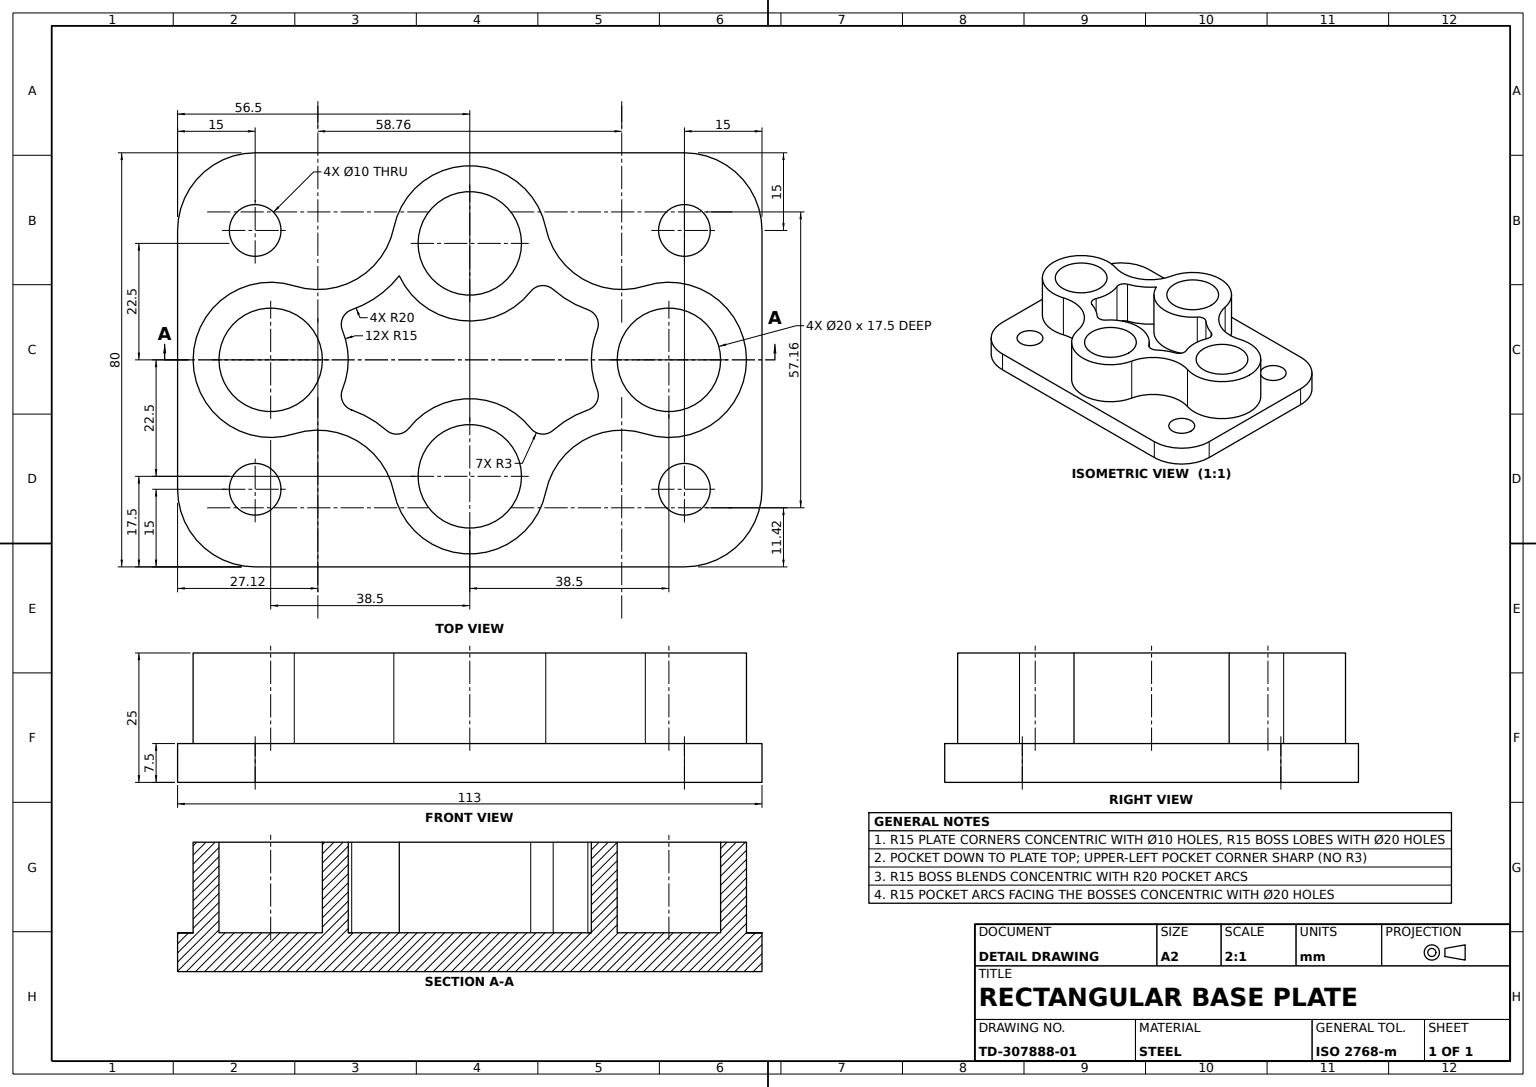
from build123d import *

# Parameters (mm, degrees)
BASE_PLATE_DEPTH            = 7.5
PORT_BOSS_SKETCH_R          = 15
QUAD_PORT_BOSS_DEPTH        = 17.5
BOSS_FILLET_R3_A_R          = 3
BOSS_FILLET_R3_B_R          = 3
BOSS_FILLET_R3_C_R          = 3
BOSS_FILLET_R3_D_R          = 3
BOSS_FILLET_R3_E_R          = 3
BOSS_FILLET_R3_F_R          = 3
BOSS_FILLET_R3_G_R          = 3
CENTRAL_CAVITY_SKETCH_R     = 10
CENTRAL_CAVITY_DEPTH        = 17.5
PLATE_CORNER_FILLET_R15_A_R = 15
PLATE_CORNER_FILLET_R15_B_R = 15
PLATE_CORNER_FILLET_R15_C_R = 15
PLATE_CORNER_FILLET_R15_D_R = 15
MOUNTING_HOLES_SKETCH_R     = 5
MOUNTING_HOLES_4X_DEPTH     = 17.5


with BuildPart() as part:
    # Base Plate Sketch → Base Plate (new body)
    with BuildSketch(Plane(origin=(0, 0, 0), x_dir=(1, 0, 0), z_dir=(0, 1, 0))):
        Polygon((40, 0), (40, 56.5), (-40, 56.5), (-40, -56.5), (40, -56.5), align=None)
    extrude(amount=BASE_PLATE_DEPTH)

    # Port Boss Sketch → Quad Port Boss (add)
    with BuildSketch(Plane(origin=(0, 7.5, 0), x_dir=(1, 0, 0), z_dir=(0, 1, 0))):
        with BuildLine():
            ThreePointArc((8.808525392, 26.35875293), (11.311943753, 19.286200894), (16.245240248, 13.633707509))
            ThreePointArc((16.245240248, 13.633707509), (20.808119068, 14.904279215), (25.539691318, 14.68878064))
            ThreePointArc((25.539691318, 14.68878064), (15.628803473, 21.809040991), (14.289691318, 33.93878064))
            ThreePointArc((14.289691318, 33.93878064), (12.155085718, 29.710580725), (8.808525392, 26.35875293))
        make_face()
        with Locations((22.5, 0)):
            Circle(PORT_BOSS_SKETCH_R)
        with BuildLine():
            ThreePointArc((8.808525392, -26.35875293), (12.155085718, -29.710580725), (14.289691318, -33.93878064))
            ThreePointArc((14.289691318, -33.93878064), (15.628803473, -21.809040991), (25.539691318, -14.68878064))
            ThreePointArc((25.539691318, -14.68878064), (20.808119068, -14.904279215), (16.245240248, -13.633707509))
            ThreePointArc((16.245240248, -13.633707509), (11.311943753, -19.286200894), (8.808525392, -26.35875293))
        make_face()
        with Locations((0, -38.5)):
            Circle(PORT_BOSS_SKETCH_R)
        with BuildLine():
            ThreePointArc((-25.539691318, -14.68878064), (-15.628803473, -21.809040991), (-14.289691318, -33.93878064))
            ThreePointArc((-14.289691318, -33.93878064), (-12.155085718, -29.710580725), (-8.808525392, -26.35875293))
            ThreePointArc((-8.808525392, -26.35875293), (-11.311943753, -19.286200894), (-16.245240248, -13.633707509))
            ThreePointArc((-16.245240248, -13.633707509), (-20.808119068, -14.904279215), (-25.539691318, -14.68878064))
        make_face()
        with Locations((-22.5, 0)):
            Circle(PORT_BOSS_SKETCH_R)
        with BuildLine():
            ThreePointArc((-14.289691318, 33.93878064), (-15.628803473, 21.809040991), (-25.539691318, 14.68878064))
            ThreePointArc((-25.539691318, 14.68878064), (-20.808119068, 14.904279215), (-16.245240248, 13.633707509))
            ThreePointArc((-16.245240248, 13.633707509), (-11.311943753, 19.286200894), (-8.808525392, 26.35875293))
            ThreePointArc((-8.808525392, 26.35875293), (-12.155085718, 29.710580725), (-14.289691318, 33.93878064))
        make_face()
        with Locations((0, 38.5)):
            Circle(PORT_BOSS_SKETCH_R)
    extrude(amount=QUAD_PORT_BOSS_DEPTH)

    # Boss Fillet R3 A
    boss_fillet_r3_a_edges = [part.edges().sort_by_distance(p)[0] for p in [
        (-8.808525392, 16.25, -26.35875293),
    ]]
    fillet(boss_fillet_r3_a_edges, radius=BOSS_FILLET_R3_A_R)

    # Boss Fillet R3 B
    boss_fillet_r3_b_edges = [part.edges().sort_by_distance(p)[0] for p in [
        (8.808525392, 16.25, -26.35875293),
    ]]
    fillet(boss_fillet_r3_b_edges, radius=BOSS_FILLET_R3_B_R)

    # Boss Fillet R3 C
    boss_fillet_r3_c_edges = [part.edges().sort_by_distance(p)[0] for p in [
        (16.245240248, 16.25, -13.633707509),
    ]]
    fillet(boss_fillet_r3_c_edges, radius=BOSS_FILLET_R3_C_R)

    # Boss Fillet R3 D
    boss_fillet_r3_d_edges = [part.edges().sort_by_distance(p)[0] for p in [
        (16.245240248, 16.25, 13.633707509),
    ]]
    fillet(boss_fillet_r3_d_edges, radius=BOSS_FILLET_R3_D_R)

    # Boss Fillet R3 E
    boss_fillet_r3_e_edges = [part.edges().sort_by_distance(p)[0] for p in [
        (-16.245240248, 16.25, -13.633707509),
    ]]
    fillet(boss_fillet_r3_e_edges, radius=BOSS_FILLET_R3_E_R)

    # Boss Fillet R3 F
    boss_fillet_r3_f_edges = [part.edges().sort_by_distance(p)[0] for p in [
        (-8.808525392, 16.25, 26.35875293),
    ]]
    fillet(boss_fillet_r3_f_edges, radius=BOSS_FILLET_R3_F_R)

    # Boss Fillet R3 G
    boss_fillet_r3_g_edges = [part.edges().sort_by_distance(p)[0] for p in [
        (8.808525392, 16.25, 26.35875293),
    ]]
    fillet(boss_fillet_r3_g_edges, radius=BOSS_FILLET_R3_G_R)

    # Central Cavity Sketch → Central Cavity (cut)
    with BuildSketch(Plane(origin=(0, 25, 0), x_dir=(1, 0, 0), z_dir=(0, 1, 0))):
        with Locations(Location((0, 38.5, 0), (0, 0, 270))):
            Circle(CENTRAL_CAVITY_SKETCH_R)
        with Locations(Location((22.5, 0, 0), (0, 0, 270))):
            Circle(CENTRAL_CAVITY_SKETCH_R)
        with Locations(Location((0, -38.5, 0), (0, 0, 270))):
            Circle(CENTRAL_CAVITY_SKETCH_R)
        with Locations(Location((-22.5, 0, 0), (0, 0, 270))):
            Circle(CENTRAL_CAVITY_SKETCH_R)
    extrude(amount=-CENTRAL_CAVITY_DEPTH, mode=Mode.SUBTRACT)

    # Plate Corner Fillet R15 A
    plate_corner_fillet_r15_a_edges = [part.edges().sort_by_distance(p)[0] for p in [
        (-40, 3.75, -56.5),
    ]]
    fillet(plate_corner_fillet_r15_a_edges, radius=PLATE_CORNER_FILLET_R15_A_R)

    # Plate Corner Fillet R15 B
    plate_corner_fillet_r15_b_edges = [part.edges().sort_by_distance(p)[0] for p in [
        (40, 3.75, -56.5),
    ]]
    fillet(plate_corner_fillet_r15_b_edges, radius=PLATE_CORNER_FILLET_R15_B_R)

    # Plate Corner Fillet R15 C
    plate_corner_fillet_r15_c_edges = [part.edges().sort_by_distance(p)[0] for p in [
        (40, 3.75, 56.5),
    ]]
    fillet(plate_corner_fillet_r15_c_edges, radius=PLATE_CORNER_FILLET_R15_C_R)

    # Plate Corner Fillet R15 D
    plate_corner_fillet_r15_d_edges = [part.edges().sort_by_distance(p)[0] for p in [
        (-40, 3.75, 56.5),
    ]]
    fillet(plate_corner_fillet_r15_d_edges, radius=PLATE_CORNER_FILLET_R15_D_R)

    # Mounting Holes Sketch → Mounting Holes 4x (cut)
    with BuildSketch(Plane(origin=(0, 7.5, 0), x_dir=(1, 0, 0), z_dir=(0, 1, 0))):
        with Locations(Location((-25, 41.5, 0), (0, 0, 270))):
            Circle(MOUNTING_HOLES_SKETCH_R)
        with Locations(Location((25, 41.5, 0), (0, 0, 270))):
            Circle(MOUNTING_HOLES_SKETCH_R)
        with Locations(Location((25, -41.5, 0), (0, 0, 270))):
            Circle(MOUNTING_HOLES_SKETCH_R)
        with Locations(Location((-25, -41.5, 0), (0, 0, 270))):
            Circle(MOUNTING_HOLES_SKETCH_R)
    extrude(amount=-MOUNTING_HOLES_4X_DEPTH, mode=Mode.SUBTRACT)


solid = part.part
